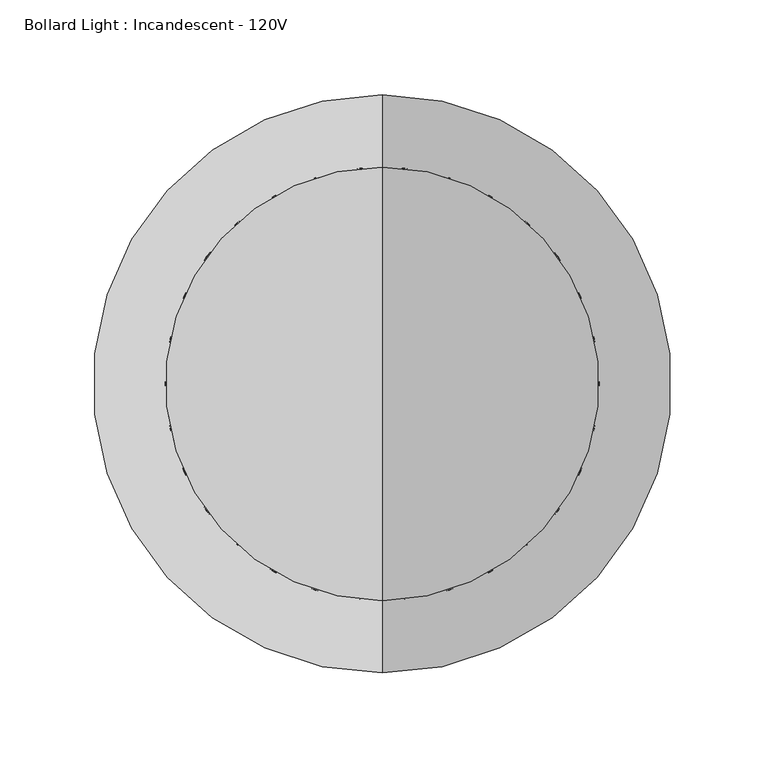
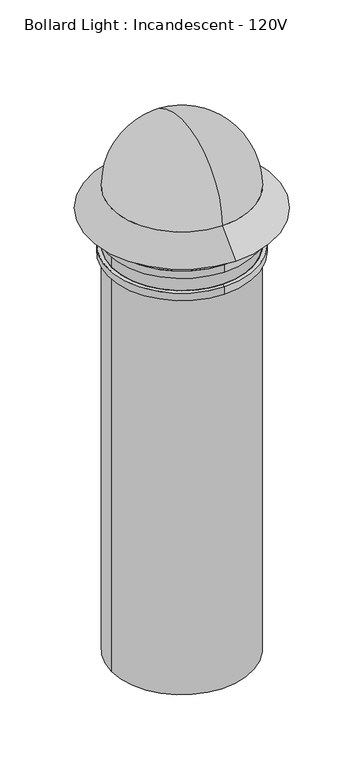
"""IFC4 building model written with IfcOpenShell, lengths in millimetres: light fixture geometry, Bollard Light : Incandescent - 120V."""

from ifc_helpers import new_model, si_unit, point, frame, frame_2d, origin, origin_with_axes, place, context, project, spatial, polyline, circle_curve, ellipse_curve, trimmed, segment, composite_curve, outline, extrude, source, transform, mapped, element, save
from ifc_brep_helpers import plane_surface, cylinder_surface, revolved_surface, advanced_brep


def bollard_light_incandescent_120v_1e792f18(model_context):
    return source(origin(), model_context, "Body", "SolidModel", [
        extrude(outline(composite_curve([segment(trimmed(circle_curve(frame_2d((-114.3, -114.3)), 114.3), [point((-228.6, -114.3))], [point((0.0, -114.3))], False, "CARTESIAN"), True, "CONTINUOUS"), segment(trimmed(circle_curve(frame_2d((-114.3, -114.3)), 114.3), [point((0.0, -114.3))], [point((-228.6, -114.3))], False, "CARTESIAN"), True, "CONTINUOUS")], self_intersect=False)), origin_with_axes(), (0.0, 0.0, 1.0), 698.5),
        advanced_brep(
        [(-114.3, -114.3, 914.4), (-114.3, 0.0, 800.1), (-114.3, -228.6, 800.1), (-114.3, -228.6, 787.4), (-114.3, 0.0, 787.4), (-114.3, -114.3, 901.7), (-114.3, -228.6, 762.0), (-114.3, 0.0, 762.0), (-114.3, -266.7, 762.0), (-114.3, 38.1, 762.0)],
        [
            (0, 1, circle_curve(frame((-114.3, -114.3, 800.1), z_axis=(-1.0, 0.0, 0.0), x_axis=(0.0, 1.0, 0.0)), 114.3)),
            (1, 2, circle_curve(frame((-114.3, -114.3, 800.1), z_axis=(0.0, 0.0, 1.0), x_axis=(0.0, 1.0, 0.0)), 114.3)),
            (2, 0, circle_curve(frame((-114.3, -114.3, 800.1), z_axis=(-1.0, 0.0, 0.0), x_axis=(0.0, -1.0, 0.0)), 114.3)),
            (2, 1, circle_curve(frame((-114.3, -114.3, 800.1), z_axis=(0.0, 0.0, 1.0), x_axis=(0.0, 1.0, 0.0)), 114.3)),
            (3, 4, circle_curve(frame((-114.3, -114.3, 787.4), z_axis=(0.0, 0.0, -1.0), x_axis=(0.0, 1.0, 0.0)), 114.3)),
            (4, 5),
            (5, 3),
            (4, 3, circle_curve(frame((-114.3, -114.3, 787.4), z_axis=(0.0, 0.0, -1.0), x_axis=(0.0, 1.0, 0.0)), 114.3)),
            (6, 7, circle_curve(frame((-114.3, -114.3, 762.0), z_axis=(0.0, 0.0, -1.0), x_axis=(0.0, 1.0, 0.0)), 114.3)),
            (7, 4),
            (3, 6),
            (7, 6, circle_curve(frame((-114.3, -114.3, 762.0), z_axis=(0.0, 0.0, -1.0), x_axis=(0.0, 1.0, 0.0)), 114.3)),
            (8, 9, circle_curve(frame((-114.3, -114.3, 762.0), z_axis=(0.0, 0.0, -1.0), x_axis=(0.0, 1.0, 0.0)), 152.4)),
            (9, 7),
            (6, 8),
            (9, 8, circle_curve(frame((-114.3, -114.3, 762.0), z_axis=(0.0, 0.0, -1.0), x_axis=(0.0, 1.0, 0.0)), 152.4)),
            (1, 9),
            (8, 2),
        ],
        [
            revolved_surface(trimmed(ellipse_curve(frame((-114.3, -114.3, 800.1), z_axis=(1.0, 0.0, 0.0), x_axis=(0.0, 1.0, 0.0)), 114.3, 114.3), [point((-114.3, 0.0, 800.1))], [point((-114.3, -114.3, 914.4))], True, "CARTESIAN"), (-114.3, -114.3, 838.2), (0.0, 0.0, 1.0)),
            revolved_surface(polyline([(-114.3, -114.3, 901.7), (-114.3, 0.0, 787.4)]), (-114.3, -114.3, 838.2), (0.0, 0.0, 1.0)),
            revolved_surface(polyline([(-114.3, 0.0, 787.4), (-114.3, 0.0, 762.0)]), (-114.3, -114.3, 838.2), (0.0, 0.0, 1.0)),
            plane_surface(frame((-114.3, -114.3, 762.0), z_axis=(0.0, 0.0, -1.0), x_axis=(0.0, 1.0, 0.0))),
            revolved_surface(polyline([(-114.3, 38.1, 762.0), (-114.3, 0.0, 800.1)]), (-114.3, -114.3, 838.2), (0.0, 0.0, 1.0)),
        ],
        [
            (0, [[1, 2, 3]]),
            (0, [[-3, 4, -1]]),
            (1, [[5, 6, 7]]),
            (1, [[8, -7, -6]]),
            (2, [[9, 10, -5, 11]]),
            (2, [[12, -11, -8, -10]]),
            (3, [[13, 14, -9, 15]]),
            (3, [[16, -15, -12, -14]]),
            (4, [[-2, 17, -13, 18]]),
            (4, [[-4, -18, -16, -17]]),
        ],
    ),
        advanced_brep(
        [(-114.3, -228.6, 698.5), (-114.3, 0.0, 698.5), (-114.3, 6.35, 698.5), (-114.3, -234.95, 698.5), (-114.3, -228.6, 685.8), (-114.3, 0.0, 685.8), (-114.3, -234.95, 685.8), (-114.3, 6.35, 685.8)],
        [
            (0, 1, circle_curve(frame((-114.3, -114.3, 698.5), z_axis=(0.0, 0.0, -1.0), x_axis=(0.0, 1.0, 0.0)), 114.3)),
            (1, 2),
            (2, 3, circle_curve(frame((-114.3, -114.3, 698.5), z_axis=(0.0, 0.0, 1.0), x_axis=(0.0, 1.0, 0.0)), 120.65)),
            (3, 0),
            (1, 0, circle_curve(frame((-114.3, -114.3, 698.5), z_axis=(0.0, 0.0, -1.0), x_axis=(0.0, 1.0, 0.0)), 114.3)),
            (3, 2, circle_curve(frame((-114.3, -114.3, 698.5), z_axis=(0.0, 0.0, 1.0), x_axis=(0.0, 1.0, 0.0)), 120.65)),
            (4, 5, circle_curve(frame((-114.3, -114.3, 685.8), z_axis=(0.0, 0.0, -1.0), x_axis=(0.0, 1.0, 0.0)), 114.3)),
            (5, 1),
            (0, 4),
            (5, 4, circle_curve(frame((-114.3, -114.3, 685.8), z_axis=(0.0, 0.0, -1.0), x_axis=(0.0, 1.0, 0.0)), 114.3)),
            (6, 7, circle_curve(frame((-114.3, -114.3, 685.8), z_axis=(0.0, 0.0, -1.0), x_axis=(0.0, 1.0, 0.0)), 120.65)),
            (7, 5),
            (4, 6),
            (7, 6, circle_curve(frame((-114.3, -114.3, 685.8), z_axis=(0.0, 0.0, -1.0), x_axis=(0.0, 1.0, 0.0)), 120.65)),
            (2, 7),
            (6, 3),
        ],
        [
            plane_surface(frame((-114.3, -114.3, 698.5), z_axis=(0.0, 0.0, 1.0), x_axis=(0.0, 1.0, 0.0))),
            revolved_surface(polyline([(-114.3, 0.0, 698.5), (-114.3, 0.0, 685.8)]), (-114.3, -114.3, 838.2), (0.0, 0.0, 1.0)),
            plane_surface(frame((-114.3, -114.3, 685.8), z_axis=(0.0, 0.0, -1.0), x_axis=(0.0, 1.0, 0.0))),
            cylinder_surface(frame((-114.3, -114.3, 838.2), z_axis=(0.0, 0.0, 1.0), x_axis=(0.0, 1.0, 0.0)), 120.65),
        ],
        [
            (0, [[1, 2, 3, 4]]),
            (0, [[5, -4, 6, -2]]),
            (1, [[7, 8, -1, 9]]),
            (1, [[10, -9, -5, -8]]),
            (2, [[11, 12, -7, 13]]),
            (2, [[14, -13, -10, -12]]),
            (3, [[-3, 15, -11, 16]]),
            (3, [[-6, -16, -14, -15]]),
        ],
    ),
        advanced_brep(
        [(-114.3, -228.6, 736.6), (-114.3, 0.0, 736.6), (-114.3, 6.35, 736.6), (-114.3, -234.95, 736.6), (-114.3, -228.6, 723.9), (-114.3, 0.0, 723.9), (-114.3, -234.95, 723.9), (-114.3, 6.35, 723.9)],
        [
            (0, 1, circle_curve(frame((-114.3, -114.3, 736.6), z_axis=(0.0, 0.0, -1.0), x_axis=(0.0, 1.0, 0.0)), 114.3)),
            (1, 2),
            (2, 3, circle_curve(frame((-114.3, -114.3, 736.6), z_axis=(0.0, 0.0, 1.0), x_axis=(0.0, 1.0, 0.0)), 120.65)),
            (3, 0),
            (1, 0, circle_curve(frame((-114.3, -114.3, 736.6), z_axis=(0.0, 0.0, -1.0), x_axis=(0.0, 1.0, 0.0)), 114.3)),
            (3, 2, circle_curve(frame((-114.3, -114.3, 736.6), z_axis=(0.0, 0.0, 1.0), x_axis=(0.0, 1.0, 0.0)), 120.65)),
            (4, 5, circle_curve(frame((-114.3, -114.3, 723.9), z_axis=(0.0, 0.0, -1.0), x_axis=(0.0, 1.0, 0.0)), 114.3)),
            (5, 1),
            (0, 4),
            (5, 4, circle_curve(frame((-114.3, -114.3, 723.9), z_axis=(0.0, 0.0, -1.0), x_axis=(0.0, 1.0, 0.0)), 114.3)),
            (6, 7, circle_curve(frame((-114.3, -114.3, 723.9), z_axis=(0.0, 0.0, -1.0), x_axis=(0.0, 1.0, 0.0)), 120.65)),
            (7, 5),
            (4, 6),
            (7, 6, circle_curve(frame((-114.3, -114.3, 723.9), z_axis=(0.0, 0.0, -1.0), x_axis=(0.0, 1.0, 0.0)), 120.65)),
            (2, 7),
            (6, 3),
        ],
        [
            plane_surface(frame((-114.3, -114.3, 736.6), z_axis=(0.0, 0.0, 1.0), x_axis=(0.0, 1.0, 0.0))),
            revolved_surface(polyline([(-114.3, 0.0, 736.6), (-114.3, 0.0, 723.9)]), (-114.3, -114.3, 838.2), (0.0, 0.0, 1.0)),
            plane_surface(frame((-114.3, -114.3, 723.9), z_axis=(0.0, 0.0, -1.0), x_axis=(0.0, 1.0, 0.0))),
            cylinder_surface(frame((-114.3, -114.3, 838.2), z_axis=(0.0, 0.0, 1.0), x_axis=(0.0, 1.0, 0.0)), 120.65),
        ],
        [
            (0, [[1, 2, 3, 4]]),
            (0, [[5, -4, 6, -2]]),
            (1, [[7, 8, -1, 9]]),
            (1, [[10, -9, -5, -8]]),
            (2, [[11, 12, -7, 13]]),
            (2, [[14, -13, -10, -12]]),
            (3, [[-3, 15, -11, 16]]),
            (3, [[-6, -16, -14, -15]]),
        ],
    ),
        extrude(outline(composite_curve([segment(trimmed(circle_curve(frame_2d((-114.3, -114.3)), 114.3), [point((-228.6, -114.3))], [point((0.0, -114.3))], False, "CARTESIAN"), True, "CONTINUOUS"), segment(trimmed(circle_curve(frame_2d((-114.3, -114.3)), 114.3), [point((0.0, -114.3))], [point((-228.6, -114.3))], False, "CARTESIAN"), True, "CONTINUOUS")], self_intersect=False), holes=[composite_curve([segment(trimmed(circle_curve(frame_2d((-114.3, -114.3)), 101.6), [point((-215.9, -114.3))], [point((-12.7, -114.3))], True, "CARTESIAN"), True, "CONTINUOUS"), segment(trimmed(circle_curve(frame_2d((-114.3, -114.3)), 101.6), [point((-12.7, -114.3))], [point((-215.9, -114.3))], True, "CARTESIAN"), True, "CONTINUOUS")], self_intersect=False)]), frame((0.0, 0.0, 698.5), z_axis=(0.0, 0.0, 1.0), x_axis=(1.0, 0.0, 0.0)), (0.0, 0.0, 1.0), 101.6),
    ])


if __name__ == "__main__":
    model = new_model("IFC4")
    model_context = context("Model", 3, world=origin())
    ifc_project = project(units=[si_unit("LENGTHUNIT", "METRE", prefix="MILLI")], contexts=[model_context])
    site = spatial("IfcSite", under=ifc_project)
    building = spatial("IfcBuilding", under=site)
    placement = place(None, origin())
    bollard_light_incandescent_120v_shape = bollard_light_incandescent_120v_1e792f18(model_context)
    element("IfcLightFixture", 1, ObjectType="Bollard Light : Incandescent - 120V", at=placement, inside=building, context=model_context, shape_type="MappedRepresentation", body=[
        mapped(bollard_light_incandescent_120v_shape, transform((0.0, 0.0, 0.0), x_axis=(1.0, 0.0, 0.0), y_axis=(0.0, 1.0, 0.0), z_axis=(0.0, 0.0, 1.0))),
    ])
    save(model, "model.ifc")

# Revit data of these elements
# Type "Bollard Light : Incandescent - 120V"
#   Lamp = "A-19"
#   Wattage = 100 W
#   built-in parameter 1150110 = 1 (stored number, unit not read)
#   built-in parameter 1114217 = 1 (stored number, unit not read)
#   built-in parameter 1150109 = 1 (stored number, unit not read)
#   built-in parameter 1150113 = 1 (stored number, unit not read)
#   Lumens = 1690 lm
#   built-in parameter 1150115 = 1 (stored number, unit not read)
#   built-in parameter 1150105 = 134.486 (stored number, unit not read)
#   Light Source Symbol Size = 2' - 0"
#   built-in parameter 1150112 = 1 (stored number, unit not read)
#   built-in parameter 1150114 = 1 (stored number, unit not read)
#   built-in parameter 1150107 = 2800 (stored number, unit not read)
#   built-in parameter 1150106 = 1.34486 (stored number, unit not read)
#   built-in parameter 1150104 = 1.57006 (stored number, unit not read)
#   Ballast Voltage = 120 V
#   built-in parameter 1114218 = 1 (stored number, unit not read)
#   built-in parameter 1150133 = 10 (stored number, unit not read)
#   Apparent Load = 100 VA
#   built-in parameter 1150134 = 4
#   built-in parameter 1150137 = 1
#   Color Filter = 16777215
#   Ballast Number of Poles = 1
#   Load Classification = Lighting - Exterior
#   Dimming Lamp Color Temperature Shift = (empty or 0)
#   Default Elevation = 0
# Element 1 (IfcLightFixture, "Bollard Light : Incandescent - 120V")
#   Materials on its faces: "Steel, Polished", "Glass", "Concrete, Precast"
# Materials
#   "Steel, Polished": class "Metal", colour RGB 247 247 247, transparency 0, Description = "Polished steel", Cost = 0
#   "Glass": class "Glass", colour RGB 0 128 192, transparency 0.75, Description = "Soda Lime Glass", Cost = 0
#   "Concrete, Precast": class "Concrete", colour RGB 198 187 187, transparency 0, Description = "Precast concrete", Cost = 0
